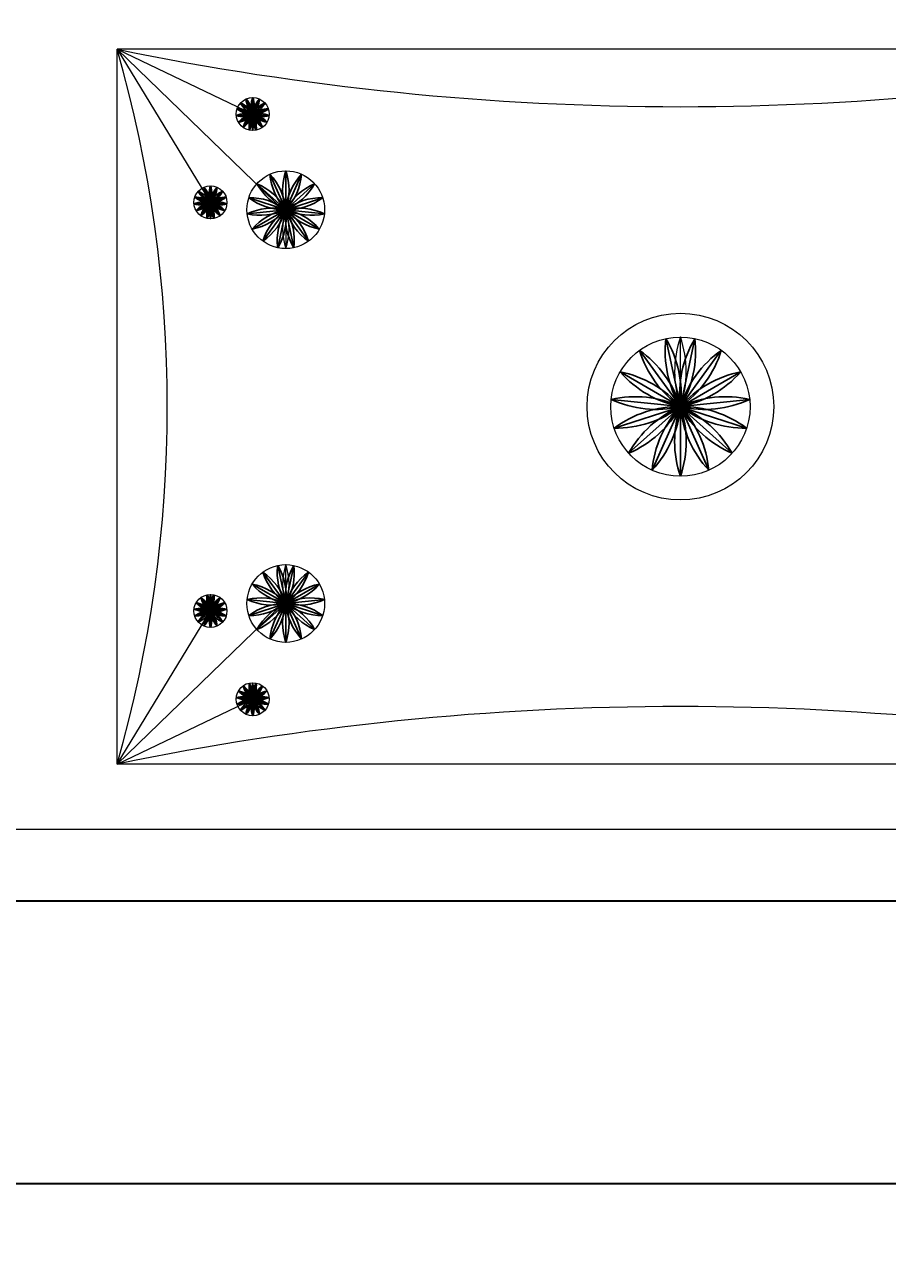
# Model space of a CAD drawing. Units: inches. Extents: x -61 to 1599, y -1316 to 257.
# Tile 36 of 204: x 134 to 152, y -790 to -763. Entities that reach past the tile are written whole.
import ezdxf

# ---------------------------------------------------------------- set-up
doc = ezdxf.new("R2010")
doc.units = ezdxf.units.IN
doc.header["$MEASUREMENT"] = 0
for name, color, linetype, lineweight in [('A-ANNO-DIMS', 2, 'Continuous', 18), ('FURNITURE', 83, 'Continuous', 18), ('WALLS', 4, 'Continuous', 35)]:
    doc.layers.add(name, color=color, linetype=linetype, lineweight=lineweight)
doc.layers.add('LT', color=8, linetype='Continuous')
doc.styles.get("Standard").update_dxf_attribs({"font": 'arial.ttf'})
doc.dimstyles.get("Standard").update_dxf_attribs({"dimtxt": 0.18, "dimasz": 0.18, "dimexe": 0.18, "dimexo": 0.0625, "dimgap": 0.09, "dimtad": 0, "dimtih": 1, "dimtoh": 1, "dimdec": 0, "dimzin": 0, "dimdsep": 46, "dimlunit": 3, "dimtxsty": 'Standard', "dimcen": 0.09, "dimadec": 0, "dimazin": 0, "dimtfac": 1, "dimtdec": 0, "dimtofl": 0, "dimtmove": 0, "dimatfit": 3, "dimfxl": 1, "dimtolj": 1, "dimtzin": 0, "dimarcsym": 0})

# ---------------------------------------------------------------- blocks, each defined once
blk = doc.blocks.new('*U3')
at = {"layer": 'LT'}
blk.add_line((0, 0.175), (0, -0.175), dxfattribs=at)
for centre, start, end in [((0.509, 0), 160.9983, 199.0017), ((-0.509, 0), 340.9983, 19.0017)]:
    blk.add_arc(centre, 0.539, start, end, dxfattribs=at)
blk = doc.blocks.new('*U4')
at = {"layer": 'LT', "transparency": 16777216}
for p, rotation in [((-66.605, -18.692), 48.00000000000001), ((-66.546, -18.649), 24), ((-66.404, -18.649), 336.0000000000001), ((-66.345, -18.692), 312), ((-66.649, -18.828), 96), ((-66.642, -18.755), 72), ((-66.627, -18.897), 120), ((-66.578, -18.951), 144), ((-66.512, -18.981), 168.0000000000001), ((-66.439, -18.981), 192), ((-66.372, -18.951), 216), ((-66.323, -18.897), 240), ((-66.308, -18.755), 288.0000000000001), ((-66.301, -18.828), 264)]:
    blk.add_blockref('*U3', p, dxfattribs=dict(at, rotation=rotation))
blk.add_blockref('*U3', (-66.475, -18.634), dxfattribs=at)
blk = doc.blocks.new('*U20')
at = {"layer": 'LT'}
blk.add_line((0, 0.175), (0, -0.175), dxfattribs=at)
for centre, start, end in [((0.509, 0), 160.9983, 199.0017), ((-0.509, 0), 340.9983, 19.0017)]:
    blk.add_arc(centre, 0.539, start, end, dxfattribs=at)
blk = doc.blocks.new('*U21')
at = {"layer": 'LT', "transparency": 16777216}
for p, rotation in [((-66.605, -18.692), 48.00000000000001), ((-66.546, -18.649), 24), ((-66.404, -18.649), 336.0000000000001), ((-66.345, -18.692), 312), ((-66.649, -18.828), 96), ((-66.642, -18.755), 72), ((-66.627, -18.897), 120), ((-66.578, -18.951), 144), ((-66.512, -18.981), 168.0000000000001), ((-66.439, -18.981), 192), ((-66.372, -18.951), 216), ((-66.323, -18.897), 240), ((-66.308, -18.755), 288.0000000000001), ((-66.301, -18.828), 264)]:
    blk.add_blockref('*U20', p, dxfattribs=dict(at, rotation=rotation))
blk.add_blockref('*U20', (-66.475, -18.634), dxfattribs=at)
blk = doc.blocks.new('*U52')
at = {"layer": 'LT'}
blk.add_line((0, 0.175), (0, -0.175), dxfattribs=at)
for centre, start, end in [((0.509, 0), 160.9983, 199.0017), ((-0.509, 0), 340.9983, 19.0017)]:
    blk.add_arc(centre, 0.539, start, end, dxfattribs=at)
blk = doc.blocks.new('*U53')
at = {"layer": 'LT', "transparency": 16777216}
for p, rotation in [((-66.605, -18.692), 48.00000000000001), ((-66.546, -18.649), 24), ((-66.404, -18.649), 336.0000000000001), ((-66.345, -18.692), 312), ((-66.649, -18.828), 96), ((-66.642, -18.755), 72), ((-66.627, -18.897), 120), ((-66.578, -18.951), 144), ((-66.512, -18.981), 168.0000000000001), ((-66.439, -18.981), 192), ((-66.372, -18.951), 216), ((-66.323, -18.897), 240), ((-66.308, -18.755), 288.0000000000001), ((-66.301, -18.828), 264)]:
    blk.add_blockref('*U52', p, dxfattribs=dict(at, rotation=rotation))
blk.add_blockref('*U52', (-66.475, -18.634), dxfattribs=at)
blk = doc.blocks.new('*U29')
at = {"layer": 'LT'}
blk.add_line((0, 0.175), (0, -0.175), dxfattribs=at)
for centre, start, end in [((0.509, 0), 160.9983, 199.0017), ((-0.509, 0), 340.9983, 19.0017)]:
    blk.add_arc(centre, 0.539, start, end, dxfattribs=at)
blk = doc.blocks.new('*U30')
at = {"layer": 'LT', "transparency": 16777216}
for p, rotation in [((-66.605, -18.692), 48.00000000000001), ((-66.546, -18.649), 24), ((-66.404, -18.649), 336.0000000000001), ((-66.345, -18.692), 312), ((-66.649, -18.828), 96), ((-66.642, -18.755), 72), ((-66.627, -18.897), 120), ((-66.578, -18.951), 144), ((-66.512, -18.981), 168.0000000000001), ((-66.439, -18.981), 192), ((-66.372, -18.951), 216), ((-66.323, -18.897), 240), ((-66.308, -18.755), 288.0000000000001), ((-66.301, -18.828), 264)]:
    blk.add_blockref('*U29', p, dxfattribs=dict(at, rotation=rotation))
blk.add_blockref('*U29', (-66.475, -18.634), dxfattribs=at)
blk = doc.blocks.new('*U5')
at = {"layer": 'LT'}
blk.add_line((0, 0.412), (0, -0.412), dxfattribs=at)
for centre, start, end in [((1.198, 0), 160.9983, 199.0017), ((-1.198, 0), 340.9983, 19.0017)]:
    blk.add_arc(centre, 1.267, start, end, dxfattribs=at)
blk = doc.blocks.new('*U47')
at = {"layer": 'LT', "transparency": 16777216}
for p, rotation in [((-156.639, -43.959), 48.00000000000001), ((-156.501, -43.858), 24), ((-156.165, -43.858), 336.0000000000001), ((-156.027, -43.959), 312), ((-156.743, -44.278), 96), ((-156.725, -44.108), 72), ((-156.69, -44.441), 120), ((-155.976, -44.441), 240), ((-155.941, -44.108), 288.0000000000001), ((-155.923, -44.278), 264), ((-156.575, -44.569), 144), ((-156.419, -44.639), 168), ((-156.247, -44.639), 192), ((-156.091, -44.569), 216)]:
    blk.add_blockref('*U5', p, dxfattribs=dict(at, rotation=rotation))
blk.add_blockref('*U5', (-156.333, -43.823), dxfattribs=at)
blk = doc.blocks.new('*U22')
at = {"layer": 'LT'}
blk.add_line((0, 0.412), (0, -0.412), dxfattribs=at)
for centre, start, end in [((1.198, 0), 160.9983, 199.0017), ((-1.198, 0), 340.9983, 19.0017)]:
    blk.add_arc(centre, 1.267, start, end, dxfattribs=at)
blk = doc.blocks.new('*U23')
at = {"layer": 'LT', "transparency": 16777216}
for p, rotation in [((-156.639, -43.959), 48.00000000000001), ((-156.501, -43.858), 24), ((-156.165, -43.858), 336.0000000000001), ((-156.027, -43.959), 312), ((-156.743, -44.278), 96), ((-156.725, -44.108), 72), ((-156.69, -44.441), 120), ((-155.976, -44.441), 240), ((-155.941, -44.108), 288.0000000000001), ((-155.923, -44.278), 264), ((-156.575, -44.569), 144), ((-156.419, -44.639), 168), ((-156.247, -44.639), 192), ((-156.091, -44.569), 216)]:
    blk.add_blockref('*U22', p, dxfattribs=dict(at, rotation=rotation))
blk.add_blockref('*U22', (-156.333, -43.823), dxfattribs=at)
blk = doc.blocks.new('*U54')
at = {"layer": 'LT'}
blk.add_line((0, 0.739), (0, -0.739), dxfattribs=at)
for centre, start, end in [((2.147, 0), 160.9983, 199.0017), ((-2.147, 0), 340.9983, 19.0017)]:
    blk.add_arc(centre, 2.27, start, end, dxfattribs=at)
blk = doc.blocks.new('*U41')
at = {"layer": 'LT', "transparency": 16777216}
blk.add_blockref('*U54', (-280.242, -78.557), dxfattribs=at)
for p, rotation in [((-280.542, -78.621), 23.99999999999999), ((-279.941, -78.621), 336.0000000000001), ((-280.791, -78.801), 48.00000000000001), ((-279.692, -78.801), 312), ((-280.945, -79.067), 72), ((-279.539, -79.067), 288.0000000000001), ((-280.977, -79.373), 96), ((-280.882, -79.665), 120), ((-280.676, -79.894), 144), ((-280.395, -80.019), 168), ((-280.088, -80.019), 191.9999999999999), ((-279.807, -79.894), 216), ((-279.602, -79.665), 240), ((-279.507, -79.373), 264)]:
    blk.add_blockref('*U54', p, dxfattribs=dict(at, rotation=rotation))
blk = doc.blocks.new('BED-DOUBLE')
for p, q in [((37.147, 1.379), (37.147, 16.557)), ((61.064, 16.557), (37.147, 16.557)), ((37.147, 16.557), (40.027, 15.18)), ((37.147, 16.557), (40.715, 13.107)), ((37.147, 16.557), (39.13, 13.305)), ((40.027, 15.18), (40.027, 14.829)), ((39.13, 13.305), (39.13, 12.955)), ((40.729, 13.149), (40.729, 12.324)), ((49.106, 8.968), (49.106, 10.447)), ((40.729, 4.788), (40.729, 5.613)), ((37.147, 1.379), (40.715, 4.83)), ((39.13, 4.631), (39.13, 4.982)), ((37.147, 1.379), (39.13, 4.631)), ((40.027, 2.756), (40.027, 3.107)), ((37.147, 1.379), (40.027, 2.756))]:
    blk.add_line(p, q)
for points in [[(1.272, 88.537), (1.272, 3.449, 0.414214), (4.722, 0), (66.813, 0, 0.414214), (70.263, 3.449), (70.263, 88.537, 0.414214), (66.813, 91.987), (4.722, 91.987, 0.414214)], [(40.027, 15.18, 0.167358), (40.027, 14.829, 0.167358)], [(39.13, 13.305, 0.167358), (39.13, 12.955, 0.167358)], [(40.729, 13.149, 0.167358), (40.729, 12.324, 0.167358)], [(49.106, 8.968, 0.167358), (49.106, 10.447, 0.167358)], [(40.729, 5.613, 0.167358), (40.729, 4.788, 0.167358)], [(39.13, 4.982, 0.167358), (39.13, 4.631, 0.167358)], [(40.027, 3.107, 0.167358), (40.027, 2.756, 0.167358)]]:
    blk.add_lwpolyline(points, format="xyb", close=True)
blk.add_lwpolyline([(61.064, 16.557), (61.064, 1.379), (37.147, 1.379)])
for centre, radius in [((40.027, 15.18), 0.351), ((40.729, 13.149), 0.825), ((39.13, 13.305), 0.351), ((49.106, 8.968), 1.982), ((49.106, 8.968), 1.478), ((40.729, 4.788), 0.825), ((39.13, 4.631), 0.351), ((40.027, 2.756), 0.351)]:
    blk.add_circle(centre, radius)
for centre, radius, start, end in [((10.674, 8.968), 27.54, 344.0046, 15.9954), ((49.106, 74.54), 59.203, 258.34678, 281.65322), ((49.106, -56.603), 59.203, 78.34678, 101.65322)]:
    blk.add_arc(centre, radius, start, end)
for name, p in [('*U30', (106.502, 33.99)), ('*U23', (197.062, 57.384)), ('*U21', (105.605, 32.115))]:
    blk.add_blockref(name, p)
at = {"rotation": 180}
blk.add_blockref('*U41', (-231.136, -70.328), dxfattribs=at)
at = {"extrusion": (0, 0, -1), "zscale": -1, "rotation": 180}
for name, p in [('*U47', (-197.062, -39.447)), ('*U4', (-105.605, -14.178)), ('*U53', (-106.502, -16.053))]:
    blk.add_blockref(name, p, dxfattribs=at)
blk = doc.blocks.new('*D687')
at = {"layer": 'A-ANNO-DIMS', "color": 0, "lineweight": -2, "transparency": 16777216}
for p, q in [((289.418, 181.677), (-61.077, 181.677)), ((-60.897, 181.497), (-60.897, -528.952)), ((-60.897, -1239.765), (-60.897, -529.316)), ((319.64, -1239.945), (-61.077, -1239.945))]:
    blk.add_line(p, q, dxfattribs=at)
at = {"layer": 'A-ANNO-DIMS', "color": 0, "transparency": 16777216}
for points in [[(-60.927, 181.497), (-60.867, 181.497), (-60.897, 181.677)], [(-60.927, -1239.765), (-60.867, -1239.765), (-60.897, -1239.945)]]:
    blk.add_solid(points, dxfattribs=at)
at = {"layer": 'DEFPOINTS', "color": 0, "transparency": 16777216}
for p in [(289.481, 181.677), (-60.897, -1239.945), (319.703, -1239.945)]:
    blk.add_point(p, dxfattribs=at)
at = {"layer": 'A-ANNO-DIMS', "color": 0, "transparency": 16777216, "insert": (-60.897, -529.134), "char_height": 0.18, "attachment_point": 5}
blk.add_mtext('\\A1;1421.6', dxfattribs=at)

msp = doc.modelspace()

# ---------------------------------------------------------------- linework, layer by layer
at = {"layer": 'WALLS'}
for p, q in [((14.7028, -781.9446), (237.7028, -781.9446)), ((14.7028, -787.9446), (237.7028, -787.9446))]:
    msp.add_line(p, q, dxfattribs=at)

# ---------------------------------------------------------------- block references
at = {"layer": 'FURNITURE'}
msp.add_blockref('BED-DOUBLE', (98.977, -780.4187), dxfattribs=at)

# ---------------------------------------------------------------- dimensions: what is measured, and where the dimension line sits
at = {"layer": 'A-ANNO-DIMS'}
dim = msp.add_linear_dim(base=(-60.8972, -1239.9446), p1=(289.4807, 181.6771), p2=(319.7028, -1239.9446), angle=90, dimstyle='Standard', override={"dimdec": 1, "dimlfac": 1, "dimrnd": 0, "dimzin": 0, "dimdsep": 46, "dimlunit": 2}, dxfattribs=at)
dim.commit()
dim.dimension.update_dxf_attribs({"geometry": '*D687', "text_midpoint": (-60.8972, -529.1337)})

doc.saveas('drawing.dxf')
